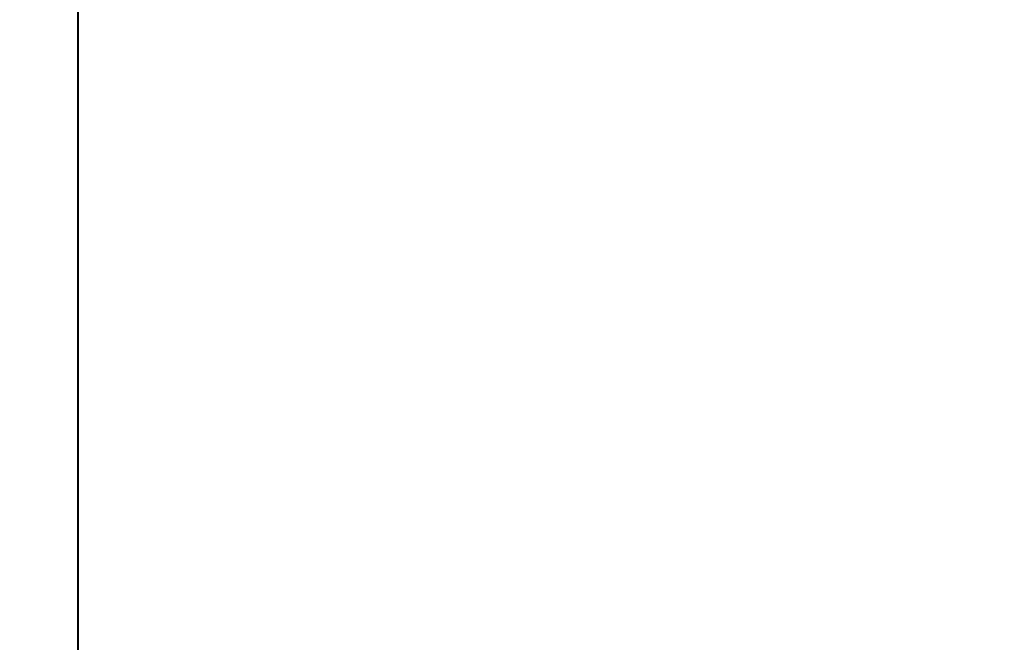
# Model space of a CAD drawing. Units: inches. Extents: x 459864 to 460310, y 324185 to 324787.
# Tile 104 of 112: x 460246.614 to 460255.113, y 324286.812 to 324292.188. Entities that reach past the tile are written whole.
import ezdxf

# ---------------------------------------------------------------- set-up
doc = ezdxf.new("R2010")
doc.units = ezdxf.units.IN
doc.layers.add('A-ANNO-DIMS', color=2, linetype='Continuous', lineweight=18)
doc.layers.add('A-WALL', color=7, linetype='Continuous', lineweight=40)
doc.styles.get("Standard").update_dxf_attribs({"font": 'arial.ttf'})
doc.dimstyles.new('ISO-25', dxfattribs={"dimtxt": 6, "dimasz": 2.5, "dimexe": 1.25, "dimexo": 0.625, "dimtad": 1, "dimdec": 1, "dimlunit": 3, "dimtxsty": 'Standard', "dimcen": 2.5, "dimadec": 0, "dimazin": 0, "dimtfac": 1, "dimtdec": 1, "dimtmove": 0, "dimatfit": 3, "dimfxl": 1, "dimarcsym": 0})

# ---------------------------------------------------------------- blocks, each defined once
blk = doc.blocks.new('*D21')
at = {"layer": 'A-ANNO-DIMS', "color": 0, "lineweight": -2, "transparency": 16777216}
for p, q in [((460247.7399, 324715.4832), (460309.5804, 324715.4832)), ((460308.3304, 324712.9832), (460308.3304, 324285.9832)), ((460247.7399, 324283.4832), (460309.5804, 324283.4832))]:
    blk.add_line(p, q, dxfattribs=at)
at = {"layer": 'A-ANNO-DIMS', "color": 0, "transparency": 16777216}
for points in [[(460307.9137, 324712.9832), (460308.747, 324712.9832), (460308.3304, 324715.4832)], [(460307.9137, 324285.9832), (460308.747, 324285.9832), (460308.3304, 324283.4832)]]:
    blk.add_solid(points, dxfattribs=at)
at = {"layer": 'Defpoints', "color": 0, "transparency": 16777216}
for p in [(460247.1149, 324715.4832), (460247.1149, 324283.4832), (460308.3304, 324283.4832)]:
    blk.add_point(p, dxfattribs=at)
at = {"layer": 'A-ANNO-DIMS', "color": 0, "transparency": 16777216, "insert": (460304.6399, 324499.4832), "char_height": 6, "attachment_point": 5, "rotation": 90}
blk.add_mtext("36'", dxfattribs=at)
blk = doc.blocks.new('*D62')
at = {"layer": 'A-ANNO-DIMS', "color": 0, "lineweight": -2, "transparency": 16777216}
for p, q in [((460247.7399, 324332.7387), (460278.7649, 324332.7387)), ((460277.5149, 324330.2387), (460277.5149, 324285.9832)), ((460247.7399, 324283.4832), (460278.7649, 324283.4832))]:
    blk.add_line(p, q, dxfattribs=at)
at = {"layer": 'A-ANNO-DIMS', "color": 0, "transparency": 16777216}
for points in [[(460277.0983, 324330.2387), (460277.9316, 324330.2387), (460277.5149, 324332.7387)], [(460277.0983, 324285.9832), (460277.9316, 324285.9832), (460277.5149, 324283.4832)]]:
    blk.add_solid(points, dxfattribs=at)
at = {"layer": 'Defpoints', "color": 0, "transparency": 16777216}
for p in [(460247.1149, 324332.7387), (460247.1149, 324283.4832), (460277.5149, 324283.4832)]:
    blk.add_point(p, dxfattribs=at)
at = {"layer": 'A-ANNO-DIMS', "color": 0, "transparency": 16777216, "insert": (460273.7876, 324308.111), "char_height": 6, "attachment_point": 5, "rotation": 90}
blk.add_mtext('4\'-1 1/2"', dxfattribs=at)
blk = doc.blocks.new('*D67')
at = {"layer": 'A-ANNO-DIMS', "color": 0, "lineweight": -2, "transparency": 16777216}
for p, q in [((460208.1149, 324284.1082), (460208.1149, 324315.1332)), ((460247.1149, 324284.1082), (460247.1149, 324315.1332)), ((460210.6149, 324313.8832), (460244.6149, 324313.8832))]:
    blk.add_line(p, q, dxfattribs=at)
at = {"layer": 'A-ANNO-DIMS', "color": 0, "transparency": 16777216}
for points in [[(460210.6149, 324314.2999), (460210.6149, 324313.4666), (460208.1149, 324313.8832)], [(460244.6149, 324314.2999), (460244.6149, 324313.4666), (460247.1149, 324313.8832)]]:
    blk.add_solid(points, dxfattribs=at)
at = {"layer": 'Defpoints', "color": 0, "transparency": 16777216}
for p in [(460247.1149, 324313.8832), (460208.1149, 324283.4832), (460247.1149, 324283.4832)]:
    blk.add_point(p, dxfattribs=at)
at = {"layer": 'A-ANNO-DIMS', "color": 0, "transparency": 16777216, "insert": (460227.6149, 324317.5737), "char_height": 6, "attachment_point": 5}
blk.add_mtext('3\'-3"', dxfattribs=at)

msp = doc.modelspace()

# ---------------------------------------------------------------- linework, layer by layer
at = {"layer": 'A-WALL'}
msp.add_line((460247.1149, 324470.9832), (460247.1149, 324283.4832), dxfattribs=at)

# ---------------------------------------------------------------- dimensions: what is measured, and where the dimension line sits
at = {"layer": 'A-ANNO-DIMS'}
for base, p1, angle, override, picture, middle in [((460308.3304, 324283.4832), (460247.1149, 324715.4832), 90, {"dimclrd": 0, "dimclre": 0, "dimclrt": 0}, '*D21', (460304.6399, 324499.4832)), ((460277.5149, 324283.4832), (460247.1149, 324332.7387), 270, {"dimdec": 1, "dimlfac": 1, "dimrnd": 0, "dimzin": 1, "dimdsep": 46, "dimlunit": 4, "dimfrac": 2}, '*D62', (460273.7876, 324308.111))]:
    dim = msp.add_linear_dim(base=base, p1=p1, p2=(460247.1149, 324283.4832), angle=angle, dimstyle='ISO-25', override=override, dxfattribs=at)
    dim.commit()
    dim.dimension.update_dxf_attribs({"geometry": picture, "text_midpoint": middle})
dim = msp.add_linear_dim(base=(460247.1149, 324313.8832), p1=(460208.1149, 324283.4832), p2=(460247.1149, 324283.4832), dimstyle='ISO-25', override={"dimdec": 1, "dimlfac": 1, "dimrnd": 0, "dimzin": 1, "dimdsep": 46, "dimlunit": 4, "dimfrac": 2}, dxfattribs=at)
dim.commit()
dim.dimension.update_dxf_attribs({"geometry": '*D67', "text_midpoint": (460227.6149, 324317.5737)})

doc.saveas('drawing.dxf')
